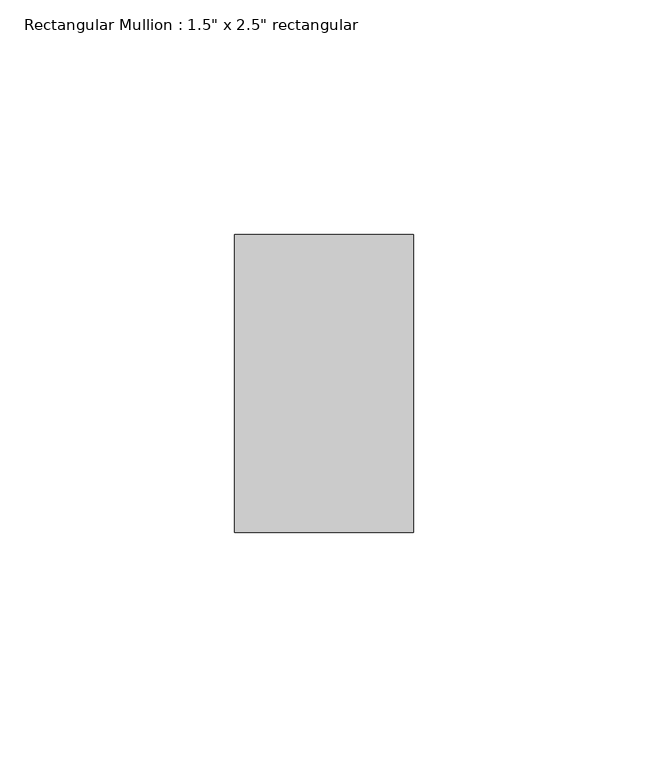
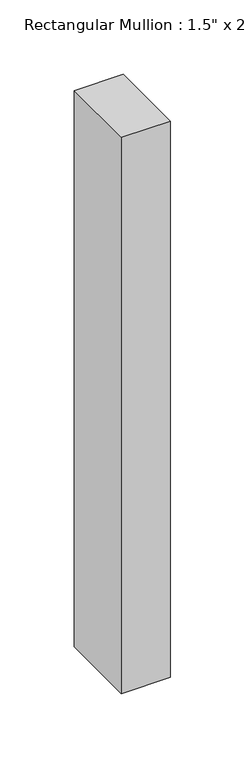
"""IFC4 building model written with IfcOpenShell, lengths in millimetres: member geometry."""

from ifc_helpers import new_model, si_unit, frame, origin, place, context, project, spatial, polyline, outline, extrude, source, transform, mapped, element, save


def member_f6fe811f(model_context):
    return source(origin(), model_context, "Body", "SweptSolid", [
        extrude(outline(polyline([(0.0, 31.75), (0.0, -31.75), (-38.1, -31.75), (-38.1, 31.75), (0.0, 31.75)])), frame((0.0, 0.0, -457.2), z_axis=(0.0, 0.0, 1.0), x_axis=(1.0, 0.0, 0.0)), (0.0, 0.0, 1.0), 457.2),
    ])


if __name__ == "__main__":
    model = new_model("IFC4")
    model_context = context("Model", 3, world=origin())
    ifc_project = project(units=[si_unit("LENGTHUNIT", "METRE", prefix="MILLI")], contexts=[model_context])
    site = spatial("IfcSite", under=ifc_project)
    building = spatial("IfcBuilding", under=site)
    placement = place(None, origin())
    member_shape = member_f6fe811f(model_context)
    element("IfcMember", 1, ObjectType="Rectangular Mullion : 1.5\" x 2.5\" rectangular", at=placement, inside=building, context=model_context, shape_type="MappedRepresentation", body=[
        mapped(member_shape, transform((0.0, 0.0, 0.0), x_axis=(1.0, 0.0, 0.0), y_axis=(0.0, 1.0, 0.0), z_axis=(0.0, 0.0, 1.0))),
    ])
    save(model, "model.ifc")

# Revit data of these elements
# Type "Rectangular Mullion : 1.5\" x 2.5\" rectangular"
#   built-in parameter 1007304 = 0.208333 (stored number, unit not read)
#   built-in parameter 1007301 = 0.0625 (stored number, unit not read)
#   built-in parameter 1007300 = 0.0625 (stored number, unit not read)
# Element 1 (IfcMember, "Rectangular Mullion : 1.5\" x 2.5\" rectangular")
#   Materials on its faces: "Leather - Black"
# Materials
#   "Leather - Black": class "Generic", colour RGB 40 40 40, transparency 0, Cost = 0
